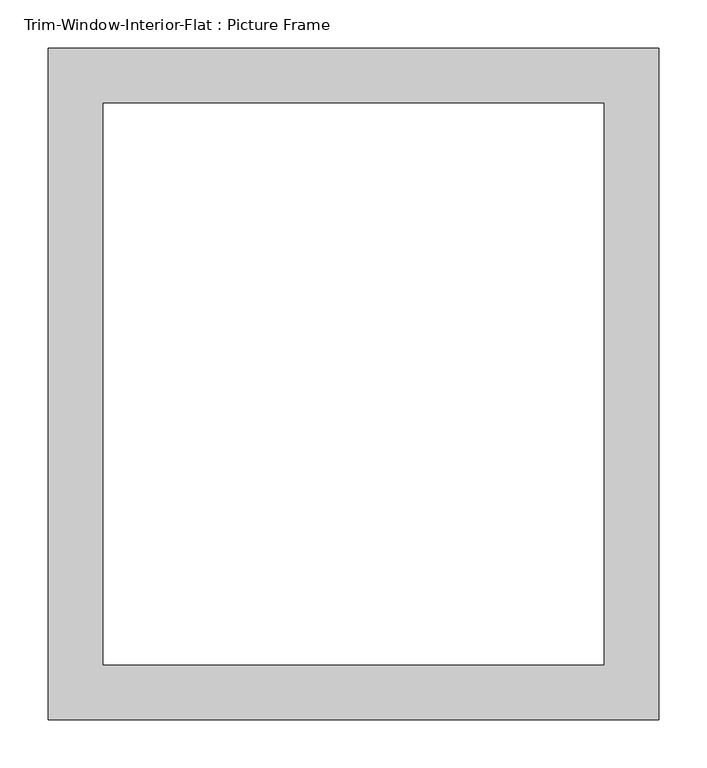
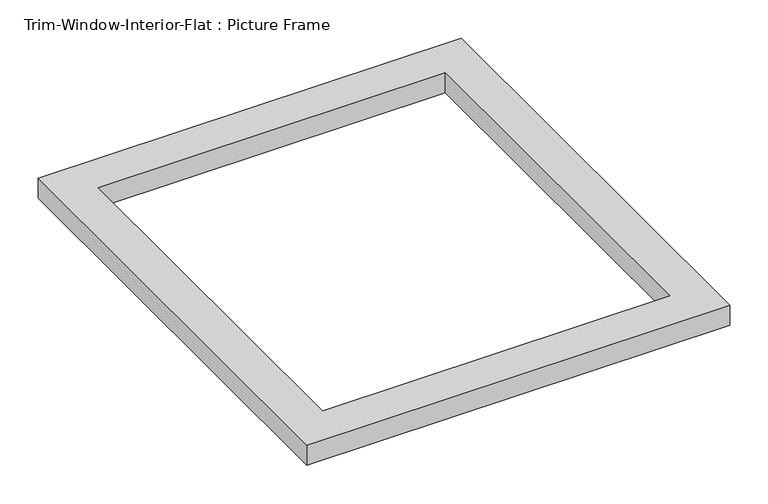
"""IFC4 building model written with IfcOpenShell, lengths in millimetres: proxy geometry, Trim-Window-Interior-Flat : Picture Frame."""

from ifc_helpers import new_model, si_unit, origin, origin_with_axes, place, context, project, spatial, polyline, outline, extrude, source, transform, mapped, element, save


def trim_window_interior_flat_picture_frame_afee5796(model_context):
    return source(origin(), model_context, "Body", "SweptSolid", [
        extrude(outline(polyline([(317.5, 44.45), (317.5, -654.05), (-317.5, -654.05), (-317.5, 44.45), (317.5, 44.45)]), holes=[polyline([(260.35, -12.7), (-260.35, -12.7), (-260.35, -596.9), (260.35, -596.9), (260.35, -12.7)])]), origin_with_axes(), (0.0, 0.0, 1.0), 31.75),
    ])


if __name__ == "__main__":
    model = new_model("IFC4")
    model_context = context("Model", 3, world=origin())
    ifc_project = project(units=[si_unit("LENGTHUNIT", "METRE", prefix="MILLI")], contexts=[model_context])
    site = spatial("IfcSite", under=ifc_project)
    building = spatial("IfcBuilding", under=site)
    placement = place(None, origin())
    trim_window_interior_flat_picture_frame_shape = trim_window_interior_flat_picture_frame_afee5796(model_context)
    element("IfcBuildingElementProxy", 1, Name="Trim-Window-Interior-Flat : Picture Frame", ObjectType="Trim-Window-Interior-Flat : Picture Frame", at=placement, inside=building, context=model_context, shape_type="MappedRepresentation", body=[
        mapped(trim_window_interior_flat_picture_frame_shape, transform((0.0, 0.0, 0.0), x_axis=(1.0, 0.0, 0.0), y_axis=(0.0, 1.0, 0.0), z_axis=(0.0, 0.0, 1.0))),
    ])
    save(model, "model.ifc")

# Revit data of these elements
# Type "Trim-Window-Interior-Flat : Picture Frame"
#   Trim Thickness_Picture Frame = 0' - 1 1/4"
#   Trim Width = 0' - 2 1/4"
#   Trim Thickness_with Sill = 0' - 0 3/4"
#   Sill Thickness = 0' - 1 1/4"
#   Opening Width [instance default] = 2' - 0"
#   Opening Height [instance default] = 3' - 0"
#   Default Elevation = 4' - 0"
#   Sill = no
#   Picture Frame = yes
#   Trim Material [instance default] = none
# Element 1 (IfcBuildingElementProxy, "Trim-Window-Interior-Flat : Picture Frame")
#   Opening Width = 1' - 9 1/2"
#   Opening Height = 2' - 0"
#   Trim Material = Wood - Stained
#   Materials on its faces: "Wood - Stained"
# Materials
#   "Wood - Stained": class "Wood", colour RGB 224 178 126, transparency 0, Cost = 0
